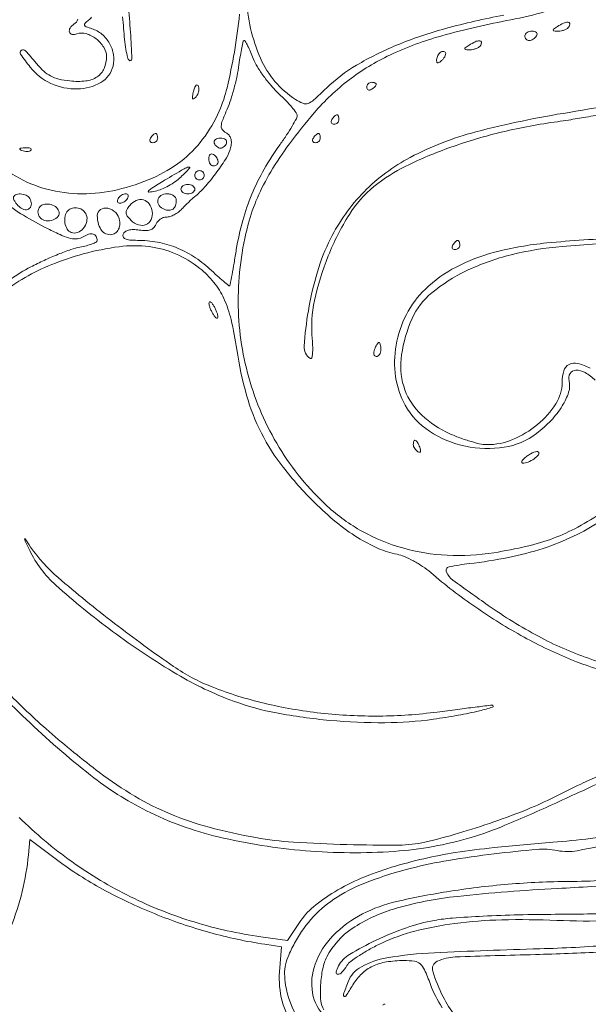
# Model space of a CAD drawing. Units: inches. Extents: x 2656 to 9931, y 1941 to 3068.
# Tile 33 of 46: x 2836.92 to 2845.52, y 2952.23 to 2967.13. Entities that reach past the tile are written whole.
import ezdxf

# ---------------------------------------------------------------- set-up
doc = ezdxf.new("R2010")
doc.units = ezdxf.units.IN
doc.layers.add('A-ANNO-DIMS', color=2, linetype='Continuous', lineweight=18)
doc.layers.add('A-ELEV-ORN', color=8, linetype='Continuous', lineweight=13)
doc.styles.get("Standard").update_dxf_attribs({"font": 'arial.ttf'})
doc.dimstyles.new('ISO-25', dxfattribs={"dimtxt": 6, "dimasz": 2.5, "dimexe": 1.25, "dimexo": 0.625, "dimtad": 1, "dimdec": 0, "dimlunit": 3, "dimtxsty": 'Standard', "dimcen": 2.5, "dimadec": 0, "dimazin": 0, "dimtfac": 1, "dimtdec": 0, "dimtmove": 0, "dimatfit": 3, "dimfxl": 1, "dimarcsym": 0})

# ---------------------------------------------------------------- blocks, each defined once
blk = doc.blocks.new('*D151')
at = {"layer": 'A-ANNO-DIMS', "color": 0, "lineweight": -2, "transparency": 16777216}
for p, q in [((2829.546, 2956.424), (2829.546, 2703.709)), ((2867.059, 2955.98), (2867.059, 2703.709)), ((2832.046, 2704.959), (2864.559, 2704.959))]:
    blk.add_line(p, q, dxfattribs=at)
at = {"layer": 'A-ANNO-DIMS', "color": 0, "transparency": 16777216}
for points in [[(2832.046, 2705.376), (2832.046, 2704.543), (2829.546, 2704.959)], [(2864.559, 2705.376), (2864.559, 2704.543), (2867.059, 2704.959)]]:
    blk.add_solid(points, dxfattribs=at)
at = {"layer": 'Defpoints', "color": 0, "transparency": 16777216}
for p in [(2829.546, 2957.049), (2867.059, 2956.605), (2867.059, 2704.959)]:
    blk.add_point(p, dxfattribs=at)
at = {"layer": 'A-ANNO-DIMS', "color": 0, "transparency": 16777216, "insert": (2848.302, 2708.689), "char_height": 6, "attachment_point": 5}
blk.add_mtext('3\'-1 1/2"', dxfattribs=at)
blk = doc.blocks.new('*D152')
at = {"layer": 'A-ANNO-DIMS', "color": 0, "lineweight": -2, "transparency": 16777216}
for p, q in [((2847.28, 2990.828), (2707.323, 2990.828)), ((2708.573, 2988.328), (2708.573, 2952.971)), ((2847.248, 2950.471), (2707.323, 2950.471))]:
    blk.add_line(p, q, dxfattribs=at)
at = {"layer": 'A-ANNO-DIMS', "color": 0, "transparency": 16777216}
for points in [[(2708.156, 2988.328), (2708.989, 2988.328), (2708.573, 2990.828)], [(2708.156, 2952.971), (2708.989, 2952.971), (2708.573, 2950.471)]]:
    blk.add_solid(points, dxfattribs=at)
at = {"layer": 'Defpoints', "color": 0, "transparency": 16777216}
for p in [(2847.905, 2990.828), (2708.573, 2950.471), (2847.873, 2950.471)]:
    blk.add_point(p, dxfattribs=at)
at = {"layer": 'A-ANNO-DIMS', "color": 0, "transparency": 16777216, "insert": (2704.843, 2970.649), "char_height": 6, "attachment_point": 5, "rotation": 90}
blk.add_mtext('3\'-4 1/2"', dxfattribs=at)
blk = doc.blocks.new('*D153')
at = {"layer": 'A-ANNO-DIMS', "color": 0, "lineweight": -2, "transparency": 16777216}
for p, q in [((2826.64, 2993.722), (2826.64, 2703.709)), ((2829.546, 2956.424), (2829.546, 2703.709)), ((2824.14, 2704.959), (2821.64, 2704.959)), ((2826.64, 2704.959), (2829.546, 2704.959)), ((2832.046, 2704.959), (2851.745, 2704.959))]:
    blk.add_line(p, q, dxfattribs=at)
at = {"layer": 'A-ANNO-DIMS', "color": 0, "transparency": 16777216}
for points in [[(2824.14, 2705.376), (2824.14, 2704.543), (2826.64, 2704.959)], [(2832.046, 2705.376), (2832.046, 2704.543), (2829.546, 2704.959)]]:
    blk.add_solid(points, dxfattribs=at)
at = {"layer": 'Defpoints', "color": 0, "transparency": 16777216}
for p in [(2826.64, 2994.347), (2829.546, 2957.049), (2829.546, 2704.959)]:
    blk.add_point(p, dxfattribs=at)
at = {"layer": 'A-ANNO-DIMS', "color": 0, "transparency": 16777216, "insert": (2843.145, 2708.65), "char_height": 6, "attachment_point": 5}
blk.add_mtext('0\'-3"', dxfattribs=at)
blk = doc.blocks.new('*D154')
at = {"layer": 'A-ANNO-DIMS', "color": 0, "lineweight": -2, "transparency": 16777216}
for p, q in [((2708.573, 2996.847), (2708.573, 2999.347)), ((2826.015, 2994.347), (2707.323, 2994.347)), ((2708.573, 2994.347), (2708.573, 2990.828)), ((2847.28, 2990.828), (2707.323, 2990.828)), ((2708.573, 2988.328), (2708.573, 2954.647))]:
    blk.add_line(p, q, dxfattribs=at)
at = {"layer": 'A-ANNO-DIMS', "color": 0, "transparency": 16777216}
for points in [[(2708.156, 2996.847), (2708.989, 2996.847), (2708.573, 2994.347)], [(2708.156, 2988.328), (2708.989, 2988.328), (2708.573, 2990.828)]]:
    blk.add_solid(points, dxfattribs=at)
at = {"layer": 'Defpoints', "color": 0, "transparency": 16777216}
for p in [(2826.64, 2994.347), (2708.573, 2990.828), (2847.905, 2990.828)]:
    blk.add_point(p, dxfattribs=at)
at = {"layer": 'A-ANNO-DIMS', "color": 0, "transparency": 16777216, "insert": (2704.843, 2970.237), "char_height": 6, "attachment_point": 5, "rotation": 90}
blk.add_mtext('0\'-3 1/2"', dxfattribs=at)

msp = doc.modelspace()

# ---------------------------------------------------------------- linework, layer by layer
at = {"layer": 'A-ELEV-ORN'}
for points in [[(2844.248, 2967.204, 0.020325), (2843.366, 2967.002, 0.031031), (2842.622, 2966.748, 0.036238), (2842.019, 2966.447, 0.058266), (2841.562, 2966.099, -0.008426), (2841.371, 2965.92, -0.09709), (2841.284, 2965.867, -0.185795), (2841.206, 2965.869, -0.048208), (2841.092, 2965.928, -0.144962), (2840.565, 2966.551, -0.095957), (2840.355, 2967.471, -0.087707)], [(2838.478, 2967.178, -0.009031), (2838.493, 2967.006, 0.010541), (2838.508, 2966.837, 0.014497), (2838.529, 2966.686, 0.01112), (2838.553, 2966.562, 0.144), (2838.576, 2966.521, 0.680381), (2838.619, 2966.54, 0.008739), (2838.598, 2966.947, 0.010925), (2838.56, 2967.362, 0.092946)], [(2840.248, 2967.219, -0.015759), (2840.169, 2966.645, -0.015384), (2840.059, 2966.106, -0.046329), (2839.94, 2965.751, -0.057689), (2839.689, 2965.324, -0.066826), (2839.357, 2964.989, -0.062657), (2838.93, 2964.738, -0.042787), (2838.396, 2964.56, -0.122852), (2837.333, 2964.57, -0.140752), (2836.461, 2965.084, -0.092959)], [(2837.801, 2967.142, -0.183925), (2837.743, 2967.066, 0.107671), (2837.684, 2967.009, 0.225328), (2837.675, 2966.948, 0.283605), (2837.716, 2966.912, 0.13417), (2837.788, 2966.919, -0.166255), (2837.925, 2966.924, -0.090422), (2838.076, 2966.847, -0.087824), (2838.194, 2966.718, -0.142734), (2838.235, 2966.577, -0.101038), (2838.198, 2966.396, -0.145814), (2838.094, 2966.27, -0.11964), (2837.921, 2966.207, -0.056254), (2837.681, 2966.207, -0.030343), (2837.513, 2966.236, -0.063936), (2837.389, 2966.283, -0.065722), (2837.283, 2966.359, -0.033711), (2837.172, 2966.478, 0.015134), (2837.01, 2966.665, 0.37613), (2836.947, 2966.672, 0.411102), (2836.936, 2966.613, 0.015349), (2837.082, 2966.415, 0.121345), (2837.394, 2966.17, 0.109947), (2837.797, 2966.086, 0.129649), (2838.148, 2966.184, 0.201375), (2838.334, 2966.433, 0.103338), (2838.341, 2966.604, 0.087789), (2838.281, 2966.774, 0.087229), (2838.165, 2966.915, 0.10013), (2838.013, 2966.999, -0.017511), (2837.928, 2967.029, -0.210796), (2837.904, 2967.054, -0.300976), (2837.91, 2967.082, -0.031957), (2837.964, 2967.128, 0.071928), (2838.009, 2967.171, 0.032471)], [(2845.748, 2959.688, -0.025269), (2845.366, 2959.454, -0.03501), (2845, 2959.287, -0.03273), (2844.597, 2959.164, -0.018565), (2844.095, 2959.067, -0.050349), (2843.389, 2959.029, -0.056473), (2842.717, 2959.138, -0.058312), (2842.106, 2959.389, -0.06025), (2841.575, 2959.772, -0.069279), (2840.847, 2960.661, -0.068805), (2840.388, 2961.718, -0.068009), (2840.228, 2962.87, -0.065125), (2840.38, 2964.041, -0.037909), (2840.517, 2964.436, -0.031231), (2840.72, 2964.833, -0.026864), (2841.002, 2965.255, -0.016079), (2841.378, 2965.725, -0.052888), (2841.904, 2966.223, -0.052742), (2842.523, 2966.6, -0.043328), (2843.31, 2966.892, -0.021083), (2844.354, 2967.133, 0.026141), (2844.873, 2967.258, 0.039837)], [(2846.868, 2966.075, -0.024075), (2845.233, 2965.732, 0.023987), (2843.821, 2965.436, 0.058336), (2842.831, 2965.051, 0.07715), (2842.131, 2964.529, 0.077589), (2841.624, 2963.819, 0.044058), (2841.426, 2963.32, 0.030707), (2841.289, 2962.729, 0.024576), (2841.225, 2962.191, 0.278284), (2841.319, 2962.008, 0.496575), (2841.34, 2962.016, 0.046305), (2841.352, 2962.08, 0.031738), (2841.355, 2962.178, 0.015856), (2841.348, 2962.303, -0.076992), (2841.382, 2962.883, -0.043013), (2841.59, 2963.559, -0.043127), (2841.909, 2964.186, -0.082003), (2842.281, 2964.609, -0.058255), (2842.766, 2964.92, -0.028484), (2843.444, 2965.204, -0.026451), (2844.231, 2965.437, -0.024677), (2845.058, 2965.591, 0.00696), (2845.225, 2965.616, 0.001918), (2845.488, 2965.66, 0.001937), (2845.785, 2965.713, 0.002024)], [(2836.676, 2964.385, 0.030498), (2836.978, 2964.174, 0.021207), (2837.343, 2963.972, 0.011172), (2837.561, 2963.869, 0.047863), (2837.697, 2963.824, 0.085233), (2837.796, 2963.818, 0.111733), (2837.881, 2963.848, -0.060682), (2837.965, 2963.887, -0.144165), (2838.033, 2963.889, -0.202373), (2838.078, 2963.855, -0.129516), (2838.094, 2963.791, -0.284283), (2838.081, 2963.769, -0.025311), (2838.017, 2963.741, -0.027039), (2837.932, 2963.714, -0.017468), (2837.831, 2963.692, 0.03803), (2837.697, 2963.656, 0.01198), (2837.504, 2963.584, 0.011889), (2837.292, 2963.492, 0.012914), (2837.09, 2963.393, 0.063336), (2836.491, 2962.974, 0.055528)], [(2836.648, 2962.986, -0.039542), (2837.002, 2963.232, -0.037445), (2837.407, 2963.429, -0.027013), (2837.883, 2963.589, -0.035466), (2838.426, 2963.699, -0.063073), (2838.881, 2963.7, -0.072275), (2839.278, 2963.591, -0.064491), (2839.646, 2963.37, -0.055043), (2839.859, 2963.159, -0.063394), (2840.01, 2962.915, -0.04983), (2840.119, 2962.596, -0.020046), (2840.206, 2962.143, 0.031606), (2840.355, 2961.449, 0.048704), (2840.578, 2960.877, 0.048617), (2840.908, 2960.359, 0.031357), (2841.381, 2959.827, 0.023668), (2841.709, 2959.531, 0.031705), (2842.034, 2959.297, 0.035791), (2842.345, 2959.132, 0.057923), (2842.631, 2959.043, -0.054429), (2842.741, 2959.01, -0.02395), (2842.878, 2958.943, -0.023362), (2843.018, 2958.858, -0.028955), (2843.14, 2958.766, 0.025593), (2843.822, 2958.24, 0.025933), (2844.552, 2957.789, 0.027491), (2845.269, 2957.445, 0.045204), (2845.91, 2957.246)], [(2846.021, 2963.83, 0.014791), (2844.896, 2963.755, 0.039833), (2844.107, 2963.615, 0.055888), (2843.524, 2963.391, 0.072546), (2843.06, 2963.057, 0.080989), (2842.772, 2962.671, 0.077086), (2842.616, 2962.208, 0.078908), (2842.609, 2961.729, 0.091687), (2842.755, 2961.298, 0.121222), (2843.121, 2960.906, 0.09198), (2843.666, 2960.679, 0.092467), (2844.253, 2960.663, 0.124359), (2844.74, 2960.871, 0.03995), (2844.962, 2961.07, 0.051287), (2845.13, 2961.288, 0.060151), (2845.227, 2961.496, 0.138403), (2845.234, 2961.668, -0.191256), (2845.249, 2961.779, -0.262948), (2845.334, 2961.829, -0.137036), (2845.477, 2961.793, -0.065835), (2845.629, 2961.677, -0.052375)], [(2845.553, 2961.859, 0.057839), (2845.366, 2961.93, 0.180103), (2845.234, 2961.916, 0.203789), (2845.154, 2961.821, 0.07515), (2845.128, 2961.645, -0.143203), (2845.033, 2961.321, -0.077515), (2844.756, 2961.007, -0.073834), (2844.379, 2960.779, -0.102152), (2843.992, 2960.703, -0.053961), (2843.875, 2960.717, -0.019026), (2843.712, 2960.761, -0.018631), (2843.535, 2960.823, -0.020788), (2843.369, 2960.896, -0.086218), (2842.96, 2961.196, -0.120227), (2842.731, 2961.586, -0.110985), (2842.699, 2962.063, -0.06598), (2842.859, 2962.611, -0.117541), (2843.155, 2963, -0.059621), (2843.677, 2963.332, -0.051554), (2844.357, 2963.577, -0.040819), (2845.128, 2963.701), (2845.655, 2963.743)], [(2846.18, 2957.3, -0.042657), (2845.525, 2957.468, -0.038553), (2844.769, 2957.801, -0.030663), (2844.009, 2958.27, -0.004), (2843.477, 2958.651, -0.130331), (2843.378, 2958.773, -0.475345), (2843.417, 2958.851, -0.026437), (2843.724, 2958.902, 0.021518), (2844.316, 2958.995, 0.028968), (2844.841, 2959.132, 0.03183), (2845.302, 2959.316, 0.03899), (2845.705, 2959.546, -0.016354)], [(2836.169, 2957.433, 0.021714), (2837.019, 2956.546, 0.024103), (2837.993, 2955.699, 0.050466), (2838.84, 2955.161, 0.058204), (2839.925, 2954.766, 0.037707), (2841.245, 2954.556, 0.037569), (2842.589, 2954.546, 0.055487), (2843.75, 2954.756, 0.026952), (2844.264, 2954.94, 0.007907), (2845.032, 2955.277, 0.002127), (2845.846, 2955.654, 0.291114)], [(2845.684, 2955.688, 0.013123), (2845.413, 2955.565, 0.004002), (2845.01, 2955.367, -0.020733), (2844.599, 2955.181, -0.012125), (2844.094, 2954.991, -0.011867), (2843.558, 2954.819, -0.014877), (2843.053, 2954.687, -0.055245), (2842.661, 2954.641, -0.008342), (2841.871, 2954.648, -0.0099), (2841.062, 2954.686, -0.027279), (2840.496, 2954.755, -0.02145), (2839.788, 2954.912, -0.03331), (2839.197, 2955.113, -0.035302), (2838.662, 2955.381, -0.028555), (2838.13, 2955.739, -0.016703), (2837.365, 2956.361, -0.021757), (2836.712, 2956.983, -0.023987)], [(2846.123, 2954.817, -0.017355), (2844.987, 2954.683, 0.004203), (2844.099, 2954.602, 0.013541), (2843.511, 2954.527, 0.018582), (2843.037, 2954.435, 0.016194), (2842.548, 2954.305, 0.027433), (2842.089, 2954.139, 0.034666), (2841.687, 2953.934, 0.038941), (2841.365, 2953.705, 0.072496), (2841.153, 2953.467), (2840.975, 2953.198), (2840.572, 2953.254, -0.040251), (2839.561, 2953.477, -0.040276), (2838.598, 2953.859, -0.040237), (2837.709, 2954.391, -0.040006), (2836.914, 2955.06, -0.026392)], [(2836.785, 2953.4, 0.03671), (2836.959, 2953.937, 0.036373), (2837.053, 2954.495), (2837.075, 2954.726), (2837.497, 2954.409, 0.036127), (2838.173, 2953.975, 0.028544), (2838.959, 2953.603, 0.028094), (2839.798, 2953.317, 0.031545), (2840.632, 2953.14), (2840.884, 2953.103), (2840.853, 2952.723, 0.086286), (2840.893, 2952.277, 0.097952), (2841.082, 2951.892, 0.097989)], [(2841.142, 2952.002, -0.100707), (2840.945, 2952.522, -0.033876), (2840.929, 2952.692, -0.062242), (2840.942, 2952.83, -0.051862), (2840.992, 2952.977, -0.017203), (2841.094, 2953.181, -0.063573), (2841.366, 2953.558, -0.063621), (2841.724, 2953.854, -0.052612), (2842.204, 2954.091, -0.026678), (2842.848, 2954.291, -0.020261), (2843.411, 2954.409, -0.011513), (2844.099, 2954.508, -0.009136), (2844.749, 2954.575, -0.070392), (2845.054, 2954.558, 0.095898), (2845.358, 2954.556, 0.010951), (2846.035, 2954.698, 0.013876)], [(2845.806, 2954.114, -0.021563), (2845.294, 2954.091, 0.019337), (2844.37, 2954.053, 0.018347), (2843.437, 2953.943, 0.018536), (2842.621, 2953.786, 0.062058), (2842.11, 2953.599, 0.080205), (2841.661, 2953.268, 0.107418), (2841.392, 2952.84, 0.130825), (2841.353, 2952.403, 0.154333), (2841.544, 2952.035, 0.024688)], [(2841.524, 2952.148, -0.129288), (2841.477, 2952.285, -0.032632), (2841.475, 2952.522, -0.034118), (2841.506, 2952.768, -0.071945), (2841.569, 2952.95, -0.126184), (2841.954, 2953.379, -0.075328), (2842.579, 2953.672, -0.045741), (2843.545, 2953.865, -0.013386), (2845.058, 2953.984, 0.008566), (2846.094, 2954.055, 0.029332)], [(2846.003, 2953.612, -0.008488), (2845.025, 2953.593, 0.005699), (2844.471, 2953.585, 0.006155), (2843.932, 2953.565, 0.006048), (2843.469, 2953.536, 0.025769), (2843.194, 2953.501, 0.040305), (2842.774, 2953.39, 0.026506), (2842.313, 2953.2, 0.023626), (2841.911, 2952.984, 0.135917), (2841.745, 2952.811, 0.062327), (2841.709, 2952.716, 0.499528), (2841.734, 2952.685, 0.205129), (2841.797, 2952.715, 0.040869), (2841.872, 2952.816, -0.092086), (2841.931, 2952.881, -0.017729), (2842.061, 2952.972, -0.01833), (2842.223, 2953.068, -0.015998), (2842.399, 2953.157, -0.046278), (2842.902, 2953.338, -0.030748), (2843.505, 2953.454, -0.026267), (2844.215, 2953.509, -0.016557), (2845.048, 2953.501, 0.017732), (2845.842, 2953.496, 0.035466)], [(2843.511, 2952.059, -0.051755), (2843.327, 2952.345, -0.041492), (2843.171, 2952.73, -0.377765), (2843.239, 2952.882, -0.098601), (2843.512, 2952.947, -0.002772), (2844.723, 2952.984, 0.007206), (2845.725, 2953.023, 0.015319), (2846.498, 2953.088, 0.019538), (2847.092, 2953.181, 0.046793), (2847.519, 2953.307, -0.030169), (2847.701, 2953.367, -0.14877), (2847.807, 2953.363, -0.147977), (2847.894, 2953.3, -0.029745), (2848.002, 2953.141, -0.023126), (2848.203, 2952.759, -0.016851), (2848.393, 2952.319, -0.01692), (2848.543, 2951.895, -0.043427)], [(2845.869, 2953.127, -0.005418), (2845.331, 2953.093, -0.005359), (2844.79, 2953.071, 0.003803), (2843.195, 2953.012, 0.031622), (2842.476, 2952.933, 0.081434), (2842.091, 2952.8, 0.17965), (2841.889, 2952.569, 0.004781), (2841.819, 2952.378, 0.361078), (2841.829, 2952.349, 0.402964), (2841.857, 2952.356, 0.004999), (2841.963, 2952.526, -0.064262), (2842.098, 2952.694, -0.080307), (2842.262, 2952.808, -0.071619), (2842.469, 2952.872, -0.040035), (2842.732, 2952.893, -0.033235), (2842.895, 2952.883, -0.149903), (2842.981, 2952.843, -0.107238), (2843.045, 2952.755, -0.013071), (2843.136, 2952.533, 0.048744), (2843.312, 2952.178, 0.037984)], [(2842.446, 2952.228, 0.51286), (2842.433, 2952.234, 0.163716), (2842.416, 2952.216, 0.010729)]]:
    msp.add_lwpolyline(points, format="xyb", dxfattribs=at)
for points in [[(2845.058, 2967.031, 0.010223), (2844.998, 2966.991, 0.295079), (2844.992, 2966.974, 0.343021), (2845.004, 2966.964, 0.012098), (2845.071, 2966.961, 0.053738), (2845.12, 2966.966, 0.049393), (2845.168, 2966.981, 0.052761), (2845.208, 2967.004, 0.101161), (2845.233, 2967.031, 0.175918), (2845.243, 2967.076, 0.372932), (2845.218, 2967.097, 0.110887), (2845.15, 2967.082, 0.03301)], [(2844.565, 2966.89, 0.092995), (2844.57, 2966.863, 0.096318), (2844.585, 2966.84, 0.099231), (2844.606, 2966.825, 0.105429), (2844.631, 2966.82, 0.089642), (2844.66, 2966.825, 0.053229), (2844.691, 2966.84, 0.051032), (2844.719, 2966.863, 0.06081), (2844.741, 2966.89, 0.139169), (2844.749, 2966.917, 0.191142), (2844.739, 2966.94, 0.138808), (2844.714, 2966.955, 0.066118), (2844.675, 2966.96, 0.062283), (2844.633, 2966.955, 0.080552), (2844.597, 2966.94, 0.097988), (2844.574, 2966.917, 0.153634)], [(2840.456, 2966.545, 0.04152), (2840.518, 2966.422, 0.020727), (2840.615, 2966.276, 0.020421), (2840.729, 2966.133, 0.028269), (2840.842, 2966.015, -0.013869), (2840.948, 2965.911, -0.018777), (2841.038, 2965.812, -0.01597), (2841.105, 2965.725, -0.158755), (2841.119, 2965.682, -0.124488), (2841.107, 2965.636, -0.009714), (2841.043, 2965.523, -0.012774), (2840.96, 2965.39, -0.009409), (2840.862, 2965.248, 0.025958), (2840.619, 2964.871, 0.031313), (2840.434, 2964.493, 0.031271), (2840.296, 2964.094, 0.02577), (2840.199, 2963.655, -0.001554), (2840.165, 2963.451, -0.002455), (2840.134, 2963.277, -0.000578), (2840.105, 2963.125, -0.103539), (2840.099, 2963.11, -0.439075), (2840.088, 2963.108, -0.002811), (2840.005, 2963.176, -0.008348), (2839.908, 2963.26, -0.004955), (2839.795, 2963.362, 0.043314), (2839.551, 2963.551, 0.04859), (2839.287, 2963.686, 0.049032), (2839.004, 2963.768, 0.04557), (2838.704, 2963.795, -0.019703), (2838.586, 2963.8, -0.081325), (2838.518, 2963.817, -0.18898), (2838.487, 2963.847, -0.199253), (2838.486, 2963.888, -0.152154), (2838.515, 2963.925, -0.087453), (2838.567, 2963.949, -0.064511), (2838.64, 2963.958, -0.034895), (2838.729, 2963.951, 0.034072), (2838.827, 2963.943, 0.08232), (2838.898, 2963.954, 0.113333), (2838.948, 2963.984, 0.108912), (2838.98, 2964.034, -0.082182), (2839.006, 2964.077, -0.065831), (2839.046, 2964.114, -0.066417), (2839.093, 2964.139, -0.087264), (2839.141, 2964.147, 0.081763), (2839.195, 2964.156, 0.039631), (2839.258, 2964.183, 0.037926), (2839.322, 2964.223, 0.044488), (2839.375, 2964.27, -0.007512), (2839.426, 2964.323, -0.005603), (2839.484, 2964.379, -0.005665), (2839.54, 2964.432, -0.012811), (2839.584, 2964.469, 0.042443), (2839.736, 2964.618, 0.020792), (2839.905, 2964.83, 0.019589), (2840.05, 2965.046, 0.07661), (2840.112, 2965.193, 0.047688), (2840.124, 2965.271, 0.08677), (2840.116, 2965.335, 0.10258), (2840.089, 2965.385, 0.090441), (2840.043, 2965.423, -0.09638), (2839.988, 2965.47, -0.183785), (2839.971, 2965.524, -0.080357), (2839.989, 2965.607, -0.009519), (2840.061, 2965.783, 0.024258), (2840.114, 2965.924, 0.01295), (2840.167, 2966.102, 0.012864), (2840.211, 2966.287, 0.019549), (2840.239, 2966.45, -0.007268), (2840.26, 2966.592, -0.011888), (2840.282, 2966.711, -0.005582), (2840.304, 2966.809, -0.348322), (2840.317, 2966.82, -0.274708), (2840.332, 2966.811, -0.007452), (2840.37, 2966.739, -0.013442), (2840.412, 2966.65, -0.008559)], [(2843.721, 2966.749, 0.010223), (2843.662, 2966.709, 0.295079), (2843.655, 2966.693, 0.343021), (2843.668, 2966.682, 0.012098), (2843.735, 2966.68, 0.053738), (2843.783, 2966.685, 0.049393), (2843.831, 2966.7, 0.052761), (2843.872, 2966.722, 0.101161), (2843.897, 2966.749, 0.175918), (2843.906, 2966.794, 0.372932), (2843.881, 2966.816, 0.110887), (2843.814, 2966.801, 0.03301)], [(2843.276, 2966.632, 0.063896), (2843.258, 2966.609, 0.039129), (2843.243, 2966.578, 0.038674), (2843.232, 2966.544, 0.054831), (2843.229, 2966.513, 0.142677), (2843.235, 2966.49, 0.290264), (2843.251, 2966.482, 0.131573), (2843.278, 2966.493, 0.034019), (2843.312, 2966.523, 0.041736), (2843.341, 2966.558, 0.061283), (2843.36, 2966.593, 0.080535), (2843.367, 2966.623, 0.212536), (2843.359, 2966.643, 0.128169), (2843.341, 2966.653, 0.100736), (2843.319, 2966.655, 0.089268), (2843.296, 2966.647, 0.075941)], [(2839.553, 2966.052, 0.013933), (2839.535, 2965.975, 0.131195), (2839.537, 2965.942, 0.470166), (2839.552, 2965.936, 0.069225), (2839.583, 2965.959, 0.0741), (2839.609, 2965.995, 0.058506), (2839.627, 2966.039, 0.059552), (2839.633, 2966.085, 0.085105), (2839.627, 2966.126, 0.170804), (2839.611, 2966.146, 0.353106), (2839.592, 2966.144, 0.106885), (2839.572, 2966.112, 0.02593)], [(2842.174, 2966.112, 0.108972), (2842.179, 2966.087, 0.182303), (2842.194, 2966.072, 0.161196), (2842.217, 2966.07, 0.082592), (2842.244, 2966.081, 0.029505), (2842.271, 2966.1, 0.035638), (2842.294, 2966.121, 0.038439), (2842.31, 2966.141, 0.151918), (2842.314, 2966.156, 0.210953), (2842.309, 2966.168, 0.081139), (2842.294, 2966.178, 0.061769), (2842.271, 2966.184, 0.042167), (2842.244, 2966.187, 0.105053), (2842.217, 2966.181, 0.099167), (2842.194, 2966.165, 0.09642), (2842.179, 2966.141, 0.093332)], [(2841.646, 2965.624, 0.082592), (2841.635, 2965.597, 0.161196), (2841.637, 2965.574, 0.182303), (2841.652, 2965.559, 0.108972), (2841.677, 2965.554, 0.093332), (2841.706, 2965.559, 0.09642), (2841.73, 2965.574, 0.099167), (2841.746, 2965.597, 0.105053), (2841.752, 2965.624, 0.042167), (2841.75, 2965.651, 0.061769), (2841.743, 2965.674, 0.081139), (2841.733, 2965.689, 0.210953), (2841.721, 2965.694, 0.151918), (2841.706, 2965.69, 0.038439), (2841.686, 2965.674, 0.035638), (2841.665, 2965.651, 0.029505)], [(2838.903, 2965.343, 0.082592), (2838.892, 2965.316, 0.161196), (2838.894, 2965.293, 0.182303), (2838.909, 2965.278, 0.108972), (2838.934, 2965.272, 0.093332), (2838.963, 2965.278, 0.09642), (2838.987, 2965.293, 0.099167), (2839.003, 2965.316, 0.105053), (2839.009, 2965.343, 0.042167), (2839.006, 2965.37, 0.061769), (2839, 2965.392, 0.081139), (2838.99, 2965.408, 0.210953), (2838.978, 2965.413, 0.151918), (2838.963, 2965.408, 0.038439), (2838.943, 2965.392, 0.035638), (2838.922, 2965.37, 0.029505)], [(2840.05, 2965.267, -0.073624), (2840.036, 2965.238, -0.066918), (2840.013, 2965.214, -0.070382), (2839.986, 2965.197, -0.102038), (2839.958, 2965.191, -0.102038), (2839.931, 2965.197, -0.070382), (2839.904, 2965.214, -0.066918), (2839.881, 2965.238, -0.073624), (2839.866, 2965.267, -0.159683), (2839.866, 2965.296, -0.143818), (2839.883, 2965.32, -0.107546), (2839.915, 2965.337, -0.064908), (2839.958, 2965.343, -0.064908), (2840.001, 2965.337, -0.107546), (2840.034, 2965.32, -0.143818), (2840.05, 2965.296, -0.159683)], [(2841.365, 2965.343, 0.082592), (2841.354, 2965.316, 0.161196), (2841.356, 2965.293, 0.182303), (2841.371, 2965.278, 0.108972), (2841.396, 2965.272, 0.093332), (2841.424, 2965.278, 0.09642), (2841.449, 2965.293, 0.099167), (2841.465, 2965.316, 0.105053), (2841.47, 2965.343, 0.042167), (2841.468, 2965.37, 0.061769), (2841.461, 2965.392, 0.081139), (2841.451, 2965.408, 0.210953), (2841.439, 2965.413, 0.151918), (2841.425, 2965.408, 0.038439), (2841.405, 2965.392, 0.035638), (2841.384, 2965.37, 0.029505)], [(2836.956, 2965.154, 0.051402), (2836.994, 2965.143, 0.05415), (2837.034, 2965.14, 0.060344), (2837.068, 2965.146, 0.126455), (2837.091, 2965.159, 0.296942), (2837.094, 2965.175, 0.208169), (2837.081, 2965.188, 0.077125), (2837.047, 2965.196, 0.028489), (2836.998, 2965.196, 0.018894), (2836.946, 2965.192, 0.168741), (2836.925, 2965.182, 0.470617), (2836.927, 2965.17, 0.054073)], [(2839.923, 2964.987, -0.105429), (2839.918, 2964.962, -0.099231), (2839.902, 2964.94, -0.096318), (2839.88, 2964.926, -0.092995), (2839.853, 2964.921, -0.153634), (2839.826, 2964.929, -0.097988), (2839.803, 2964.953, -0.080552), (2839.788, 2964.988, -0.062283), (2839.782, 2965.03, -0.066118), (2839.788, 2965.069, -0.138808), (2839.803, 2965.095, -0.191142), (2839.826, 2965.104, -0.139169), (2839.853, 2965.096, -0.06081), (2839.88, 2965.075, -0.051032), (2839.902, 2965.046, -0.053229), (2839.918, 2965.015, -0.089642)], [(2839.359, 2964.753, -0.038721), (2839.277, 2964.686, -0.026099), (2839.174, 2964.621, -0.026336), (2839.067, 2964.569, -0.046401), (2838.974, 2964.54, -0.029616), (2838.879, 2964.525, -0.675796), (2838.87, 2964.542, -0.077167), (2838.921, 2964.586, -0.003739), (2839.114, 2964.704, -0.002304), (2839.408, 2964.877, -0.082346), (2839.482, 2964.905, -0.734629), (2839.492, 2964.887, -0.010593)], [(2839.712, 2964.78, -0.099038), (2839.707, 2964.753, -0.097945), (2839.691, 2964.73, -0.097945), (2839.669, 2964.715, -0.099038), (2839.642, 2964.71, -0.099038), (2839.615, 2964.715, -0.097945), (2839.592, 2964.73, -0.097945), (2839.577, 2964.753, -0.099038), (2839.571, 2964.78, -0.099038), (2839.577, 2964.807, -0.097945), (2839.592, 2964.83, -0.097945), (2839.615, 2964.845, -0.099038), (2839.642, 2964.85, -0.099038), (2839.669, 2964.845, -0.097945), (2839.691, 2964.83, -0.097945), (2839.707, 2964.807, -0.099038)], [(2839.571, 2964.569, -0.148195), (2839.563, 2964.542, -0.098894), (2839.54, 2964.519, -0.082425), (2839.506, 2964.504, -0.064853), (2839.466, 2964.499, -0.064853), (2839.426, 2964.504, -0.082425), (2839.391, 2964.519, -0.098894), (2839.369, 2964.542, -0.148195), (2839.36, 2964.569, -0.148195), (2839.369, 2964.596, -0.098894), (2839.391, 2964.619, -0.082425), (2839.426, 2964.634, -0.064853), (2839.466, 2964.639, -0.064853), (2839.506, 2964.634, -0.082425), (2839.54, 2964.619, -0.098894), (2839.563, 2964.596, -0.148195)], [(2837.075, 2964.428, -0.133358), (2837.099, 2964.346, -0.215554), (2837.071, 2964.28, -0.223994), (2837.004, 2964.259, -0.139938), (2836.928, 2964.293, -0.033484), (2836.89, 2964.329, -0.035275), (2836.858, 2964.369, -0.037707), (2836.835, 2964.408, -0.113581), (2836.828, 2964.437, -0.291763), (2836.857, 2964.482, -0.118104), (2836.931, 2964.497, -0.094142), (2837.018, 2964.477, -0.152872)], [(2838.552, 2964.428, -0.064269), (2838.53, 2964.401, -0.051777), (2838.5, 2964.379, -0.053414), (2838.468, 2964.363, -0.085235), (2838.438, 2964.358, -0.117858), (2838.414, 2964.364, -0.186277), (2838.401, 2964.379, -0.154201), (2838.4, 2964.401, -0.076764), (2838.411, 2964.428, -0.064269), (2838.433, 2964.455, -0.051777), (2838.462, 2964.478, -0.053414), (2838.495, 2964.493, -0.085235), (2838.525, 2964.499, -0.117858), (2838.548, 2964.493, -0.186277), (2838.562, 2964.478, -0.154201), (2838.563, 2964.455, -0.076764)], [(2839.29, 2964.405, -0.071951), (2839.278, 2964.321, -0.158715), (2839.242, 2964.269, -0.170852), (2839.184, 2964.25, -0.086065), (2839.107, 2964.265, -0.142098), (2839.031, 2964.323, -0.207321), (2839.012, 2964.403, -0.20873), (2839.058, 2964.472, -0.143413), (2839.149, 2964.499, -0.064853), (2839.203, 2964.492, -0.082425), (2839.249, 2964.471, -0.098894), (2839.279, 2964.441, -0.148195)], [(2837.514, 2964.235, -0.249378), (2837.502, 2964.16, -0.140064), (2837.426, 2964.104, -0.117741), (2837.321, 2964.091, -0.170266), (2837.238, 2964.132, -0.08302), (2837.213, 2964.166, -0.075174), (2837.2, 2964.207, -0.077648), (2837.2, 2964.249, -0.099717), (2837.214, 2964.285, -0.179958), (2837.278, 2964.335, -0.118434), (2837.373, 2964.342, -0.113816), (2837.463, 2964.305, -0.158698)], [(2838.926, 2964.234, -0.136408), (2838.91, 2964.111, -0.195277), (2838.833, 2964.034, -0.180263), (2838.718, 2964.029, -0.118248), (2838.605, 2964.099, -0.035488), (2838.55, 2964.162, -0.141058), (2838.531, 2964.21, -0.151844), (2838.542, 2964.259, -0.043258), (2838.586, 2964.322, -0.1134), (2838.686, 2964.398, -0.171983), (2838.793, 2964.408, -0.176384), (2838.881, 2964.347, -0.119535)], [(2837.929, 2964.181, -0.152311), (2837.935, 2964.078, -0.115895), (2837.884, 2963.976, -0.124329), (2837.796, 2963.913, -0.187842), (2837.702, 2963.913, -0.169501), (2837.64, 2963.965, -0.09309), (2837.606, 2964.06, -0.090495), (2837.608, 2964.164, -0.147527), (2837.649, 2964.241, -0.132848), (2837.719, 2964.281, -0.117217), (2837.804, 2964.283, -0.117202), (2837.881, 2964.247, -0.132791)], [(2838.433, 2964.094, -0.060398), (2838.435, 2964.025, -0.084266), (2838.418, 2963.966, -0.094427), (2838.386, 2963.92, -0.098135), (2838.338, 2963.89, -0.160556), (2838.248, 2963.886, -0.147146), (2838.169, 2963.936, -0.110248), (2838.115, 2964.036, -0.067198), (2838.095, 2964.169, -0.251777), (2838.143, 2964.26, -0.205972), (2838.253, 2964.281, -0.144715), (2838.374, 2964.214, -0.160086)], [(2843.475, 2963.725, 0.082592), (2843.464, 2963.698, 0.161196), (2843.466, 2963.675, 0.182303), (2843.481, 2963.66, 0.108972), (2843.506, 2963.655, 0.093332), (2843.534, 2963.66, 0.09642), (2843.559, 2963.675, 0.099167), (2843.575, 2963.698, 0.105053), (2843.58, 2963.725, 0.042167), (2843.578, 2963.752, 0.061769), (2843.571, 2963.775, 0.081139), (2843.561, 2963.79, 0.210953), (2843.549, 2963.795, 0.151918), (2843.535, 2963.791, 0.038439), (2843.515, 2963.775, 0.035638), (2843.494, 2963.752, 0.029505)], [(2839.785, 2962.846, 0.067616), (2839.789, 2962.812, 0.024967), (2839.805, 2962.765, 0.024204), (2839.827, 2962.716, 0.026766), (2839.853, 2962.67, 0.027796), (2839.879, 2962.634, 0.102785), (2839.901, 2962.616, 0.335455), (2839.914, 2962.618, 0.190341), (2839.921, 2962.635, 0.067616), (2839.916, 2962.669, 0.024967), (2839.901, 2962.715, 0.024204), (2839.879, 2962.765, 0.026766), (2839.853, 2962.811, 0.027796), (2839.826, 2962.847, 0.102785), (2839.805, 2962.864, 0.335455), (2839.791, 2962.862, 0.190341)], [(2842.289, 2962.142, 0.055937), (2842.279, 2962.102, 0.100118), (2842.28, 2962.068, 0.147206), (2842.294, 2962.046, 0.184534), (2842.317, 2962.037, 0.152681), (2842.343, 2962.045, 0.098158), (2842.365, 2962.068, 0.08088), (2842.38, 2962.102, 0.062722), (2842.385, 2962.142, 0.024748), (2842.383, 2962.183, 0.039339), (2842.377, 2962.217, 0.046727), (2842.368, 2962.241, 0.289661), (2842.357, 2962.248, 0.222225), (2842.344, 2962.242, 0.030693), (2842.326, 2962.217, 0.030395), (2842.307, 2962.183, 0.02136)], [(2842.877, 2960.705, 0.088797), (2842.882, 2960.676, 0.053277), (2842.898, 2960.645, 0.051183), (2842.92, 2960.617, 0.061454), (2842.947, 2960.596, 0.1144), (2842.97, 2960.588, 0.32948), (2842.984, 2960.596, 0.155351), (2842.987, 2960.621, 0.036408), (2842.974, 2960.662, 0.029964), (2842.94, 2960.737, 0.168622), (2842.908, 2960.767, 0.444011), (2842.885, 2960.757, 0.079093)], [(2844.595, 2960.526, 0.023861), (2844.548, 2960.487, 0.066699), (2844.52, 2960.453, 0.205107), (2844.517, 2960.433, 0.338728), (2844.53, 2960.423, 0.103287), (2844.613, 2960.438, 0.054406), (2844.705, 2960.489, 0.063301), (2844.771, 2960.549, 0.390949), (2844.769, 2960.591, 0.237089), (2844.745, 2960.598, 0.05216), (2844.702, 2960.587, 0.043644), (2844.65, 2960.563, 0.029758)], [(2837.074, 2959.102, 0.099244), (2837.468, 2958.575, 0.023432), (2838.326, 2957.876, 0.025081), (2839.301, 2957.227, 0.046577), (2840.158, 2956.82, 0.041429), (2840.809, 2956.641, 0.023697), (2841.615, 2956.529, 0.02347), (2842.448, 2956.493, 0.034254), (2843.18, 2956.546, 0.0092), (2843.554, 2956.606, 0.013553), (2843.879, 2956.674, 0.022898), (2844.076, 2956.73, 0.803803), (2844.073, 2956.757, 0.057534), (2844.046, 2956.757, 0.000394), (2843.813, 2956.729, 0.001537), (2843.548, 2956.695, 0.000982), (2843.239, 2956.655, -0.03077), (2842.363, 2956.594, -0.029796), (2841.477, 2956.639, -0.030389), (2840.621, 2956.788, -0.03567), (2839.835, 2957.034, -0.056979), (2839.249, 2957.345, -0.013579), (2838.356, 2957.996, -0.01315), (2837.502, 2958.692, -0.064512), (2837.087, 2959.153, 0.000752), (2837.002, 2959.277, 0.641464), (2836.996, 2959.276, 0.175805), (2836.997, 2959.263, 0.000459)]]:
    msp.add_lwpolyline(points, format="xyb", close=True, dxfattribs=at)

# ---------------------------------------------------------------- dimensions: what is measured, and where the dimension line sits
at = {"layer": 'A-ANNO-DIMS'}
for base, p1, p2, picture, middle in [((2708.573, 2990.828), (2826.64, 2994.347), (2847.905, 2990.828), '*D154', (2704.843, 2970.237)), ((2708.573, 2950.471), (2847.905, 2990.828), (2847.873, 2950.471), '*D152', (2704.843, 2970.649))]:
    dim = msp.add_linear_dim(base=base, p1=p1, p2=p2, angle=90, dimstyle='ISO-25', override={"dimdec": 1, "dimlfac": 1, "dimrnd": 0, "dimzin": 1, "dimdsep": 46, "dimlunit": 4, "dimfrac": 2}, dxfattribs=at)
    dim.commit()
    dim.dimension.update_dxf_attribs({"geometry": picture, "text_midpoint": middle})
for base, p1, p2, picture, middle in [((2829.546, 2704.959), (2826.64, 2994.347), (2829.546, 2957.049), '*D153', (2843.145, 2708.65)), ((2867.059, 2704.959), (2829.546, 2957.049), (2867.059, 2956.605), '*D151', (2848.302, 2708.689))]:
    dim = msp.add_linear_dim(base=base, p1=p1, p2=p2, dimstyle='ISO-25', override={"dimdec": 1, "dimlfac": 1, "dimrnd": 0, "dimzin": 1, "dimdsep": 46, "dimlunit": 4, "dimfrac": 2}, dxfattribs=at)
    dim.commit()
    dim.dimension.update_dxf_attribs({"geometry": picture, "text_midpoint": middle})

doc.saveas('drawing.dxf')
